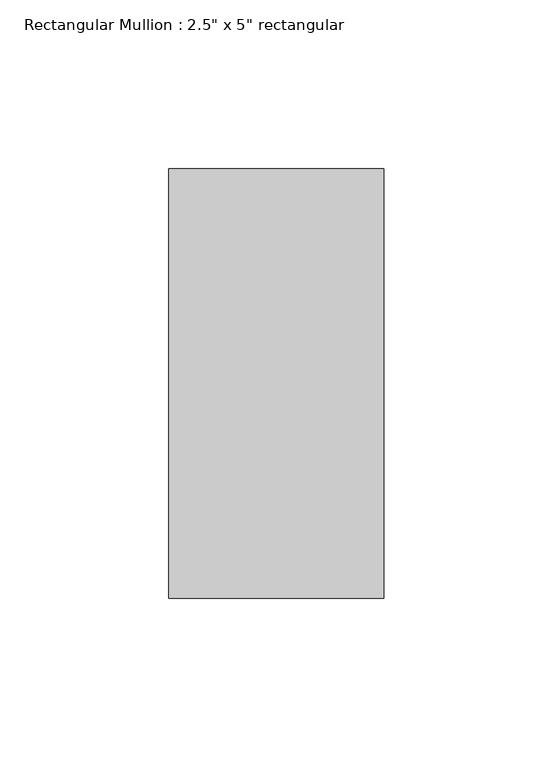
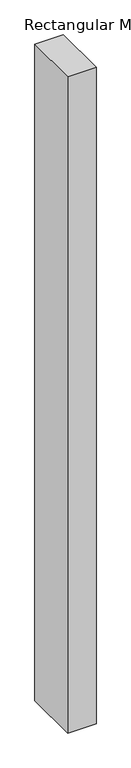
"""IFC4 building model written with IfcOpenShell, lengths in millimetres: member geometry."""

from ifc_helpers import new_model, si_unit, frame, origin, place, context, project, spatial, polyline, outline, extrude, source, transform, mapped, element, save


def member_5ff6c43e(model_context):
    return source(origin(), model_context, "Body", "SweptSolid", [
        extrude(outline(polyline([(31.75, 63.5), (31.75, -63.5), (-31.75, -63.5), (-31.75, 63.5), (31.75, 63.5)])), frame((0.0, 0.0, -1553.4572054), z_axis=(0.0, 0.0, 1.0), x_axis=(1.0, 0.0, 0.0)), (0.0, 0.0, 1.0), 1553.4572054),
    ])


if __name__ == "__main__":
    model = new_model("IFC4")
    model_context = context("Model", 3, world=origin())
    ifc_project = project(units=[si_unit("LENGTHUNIT", "METRE", prefix="MILLI")], contexts=[model_context])
    site = spatial("IfcSite", under=ifc_project)
    building = spatial("IfcBuilding", under=site)
    placement = place(None, origin())
    member_shape = member_5ff6c43e(model_context)
    element("IfcMember", 1, ObjectType="Rectangular Mullion : 2.5\" x 5\" rectangular", at=placement, inside=building, context=model_context, shape_type="MappedRepresentation", body=[
        mapped(member_shape, transform((0.0, 0.0, 0.0), x_axis=(1.0, 0.0, 0.0), y_axis=(0.0, 1.0, 0.0), z_axis=(0.0, 0.0, 1.0))),
    ])
    save(model, "model.ifc")

# Revit data of these elements
# Type "Rectangular Mullion : 2.5\" x 5\" rectangular"
#   built-in parameter 1007304 = 0.416667 (stored number, unit not read)
#   built-in parameter 1007301 = 0.104167 (stored number, unit not read)
#   built-in parameter 1007300 = 0.104167 (stored number, unit not read)
# Element 1 (IfcMember, "Rectangular Mullion : 2.5\" x 5\" rectangular")
#   Materials on its faces: "Aluminum"
# Materials
#   "Aluminum": class "Metal", colour RGB 247 247 247, transparency 0, Description = "Aluminum 6061", Cost = 0
